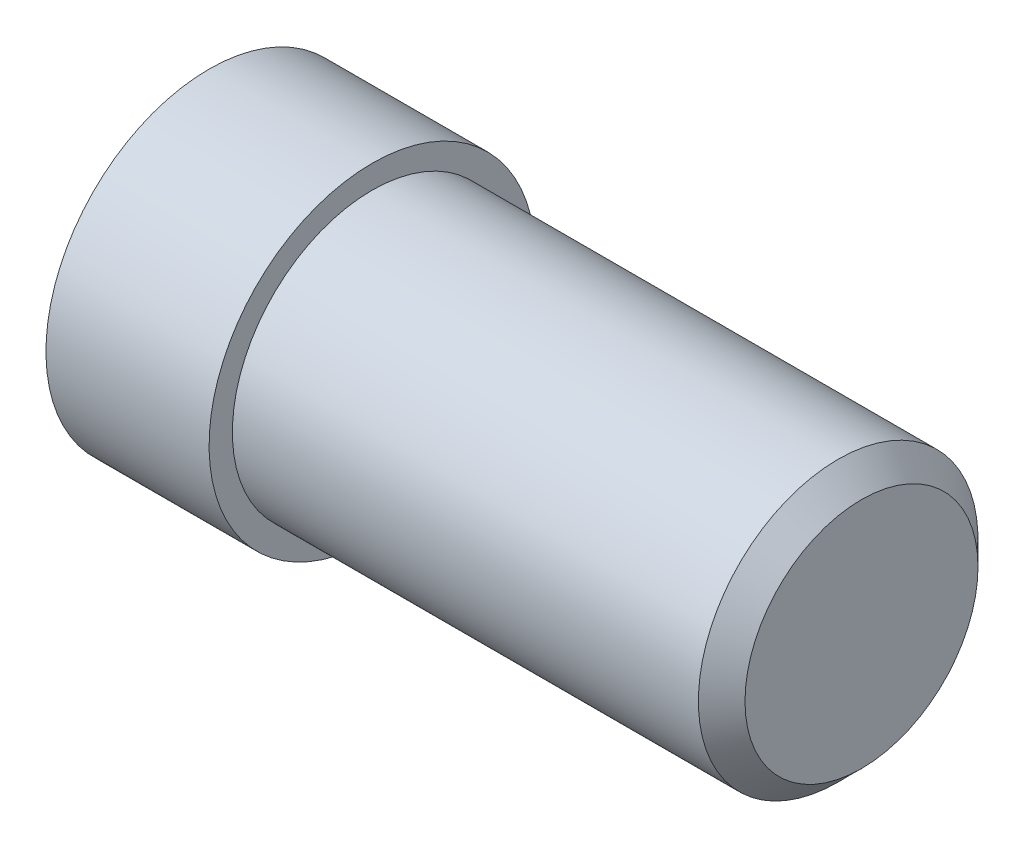
ISO-10303-21;
HEADER;
FILE_DESCRIPTION(('STEP AP214'),'2;1');
FILE_NAME('part.step','',(''),(''),'','','');
FILE_SCHEMA(('AUTOMOTIVE_DESIGN { 1 0 10303 214 1 1 1 1 }'));
ENDSEC;
DATA;
#1=APPLICATION_CONTEXT('core data for automotive mechanical design processes');
#2=APPLICATION_PROTOCOL_DEFINITION('international standard','automotive_design',2000,#1);
#3=PRODUCT_CONTEXT('',#1,'mechanical');
#4=PRODUCT('Part','Part','',(#3));
#5=PRODUCT_RELATED_PRODUCT_CATEGORY('part','',(#4));
#6=PRODUCT_DEFINITION_FORMATION('','',#4);
#7=PRODUCT_DEFINITION_CONTEXT('part definition',#1,'design');
#8=PRODUCT_DEFINITION('design','',#6,#7);
#9=PRODUCT_DEFINITION_SHAPE('','',#8);
#10=(LENGTH_UNIT() NAMED_UNIT(*) SI_UNIT(.MILLI.,.METRE.));
#11=(NAMED_UNIT(*) PLANE_ANGLE_UNIT() SI_UNIT($,.RADIAN.));
#12=(NAMED_UNIT(*) SI_UNIT($,.STERADIAN.) SOLID_ANGLE_UNIT());
#13=UNCERTAINTY_MEASURE_WITH_UNIT(LENGTH_MEASURE(1.E-05),#10,'distance_accuracy_value','');
#14=(GEOMETRIC_REPRESENTATION_CONTEXT(3) GLOBAL_UNCERTAINTY_ASSIGNED_CONTEXT((#13)) GLOBAL_UNIT_ASSIGNED_CONTEXT((#10,
#11,#12)) REPRESENTATION_CONTEXT('',''));
#15=CARTESIAN_POINT('',(0.,0.,0.));
#16=DIRECTION('',(0.,0.,1.));
#17=DIRECTION('',(1.,0.,0.));
#18=AXIS2_PLACEMENT_3D('',#15,#16,#17);
#19=CARTESIAN_POINT('',(0.,0.,0.));
#20=DIRECTION('',(1.,0.,0.));
#21=DIRECTION('',(0.,1.,0.));
#22=AXIS2_PLACEMENT_3D('',#19,#20,#21);
#23=PLANE('',#22);
#24=CARTESIAN_POINT('',(0.,0.,0.));
#25=DIRECTION('',(1.,0.,0.));
#26=DIRECTION('',(0.,1.,0.));
#27=AXIS2_PLACEMENT_3D('',#24,#25,#26);
#28=CIRCLE('',#27,5.);
#29=CARTESIAN_POINT('',(0.,5.,0.));
#30=VERTEX_POINT('',#29);
#31=EDGE_CURVE('E50',#30,#30,#28,.T.);
#32=ORIENTED_EDGE('',*,*,#31,.T.);
#33=EDGE_LOOP('',(#32));
#34=FACE_BOUND('',#33,.T.);
#35=ADVANCED_FACE('F39',(#34),#23,.T.);
#36=CARTESIAN_POINT('',(0.,0.,0.));
#37=DIRECTION('',(1.,0.,0.));
#38=DIRECTION('',(0.,1.,0.));
#39=AXIS2_PLACEMENT_3D('',#36,#37,#38);
#40=CYLINDRICAL_SURFACE('',#39,6.);
#41=CARTESIAN_POINT('',(-1.,0.,0.));
#42=DIRECTION('',(1.,0.,0.));
#43=DIRECTION('',(0.,1.,0.));
#44=AXIS2_PLACEMENT_3D('',#41,#42,#43);
#45=CIRCLE('',#44,6.);
#46=CARTESIAN_POINT('',(-1.,6.,0.));
#47=VERTEX_POINT('',#46);
#48=EDGE_CURVE('E10',#47,#47,#45,.F.);
#49=ORIENTED_EDGE('',*,*,#48,.T.);
#50=EDGE_LOOP('',(#49));
#51=FACE_BOUND('',#50,.T.);
#52=CARTESIAN_POINT('',(-21.,0.,0.));
#53=DIRECTION('',(1.,0.,0.));
#54=DIRECTION('',(0.,1.,0.));
#55=AXIS2_PLACEMENT_3D('',#52,#53,#54);
#56=CIRCLE('',#55,6.);
#57=CARTESIAN_POINT('',(-21.,5.99999999999999,0.));
#58=VERTEX_POINT('',#57);
#59=EDGE_CURVE('E51',#58,#58,#56,.T.);
#60=ORIENTED_EDGE('',*,*,#59,.T.);
#61=EDGE_LOOP('',(#60));
#62=FACE_BOUND('',#61,.T.);
#63=ADVANCED_FACE('F76',(#51,#62),#40,.T.);
#64=CARTESIAN_POINT('',(-21.,5.99999999999999,0.));
#65=DIRECTION('',(1.,0.,0.));
#66=DIRECTION('',(0.,1.,0.));
#67=AXIS2_PLACEMENT_3D('',#64,#65,#66);
#68=PLANE('',#67);
#69=CARTESIAN_POINT('',(-21.,0.,0.));
#70=DIRECTION('',(1.,0.,0.));
#71=DIRECTION('',(0.,1.,0.));
#72=AXIS2_PLACEMENT_3D('',#69,#70,#71);
#73=CIRCLE('',#72,7.);
#74=CARTESIAN_POINT('',(-21.,7.,0.));
#75=VERTEX_POINT('',#74);
#76=EDGE_CURVE('E54',#75,#75,#73,.T.);
#77=ORIENTED_EDGE('',*,*,#76,.T.);
#78=EDGE_LOOP('',(#77));
#79=FACE_BOUND('',#78,.T.);
#80=ORIENTED_EDGE('',*,*,#59,.F.);
#81=EDGE_LOOP('',(#80));
#82=FACE_BOUND('',#81,.T.);
#83=ADVANCED_FACE('F77',(#79,#82),#68,.T.);
#84=CARTESIAN_POINT('',(0.,0.,0.));
#85=DIRECTION('',(1.,0.,0.));
#86=DIRECTION('',(0.,1.,0.));
#87=AXIS2_PLACEMENT_3D('',#84,#85,#86);
#88=CYLINDRICAL_SURFACE('',#87,7.);
#89=CARTESIAN_POINT('',(-28.,0.,0.));
#90=DIRECTION('',(1.,0.,0.));
#91=DIRECTION('',(0.,1.,0.));
#92=AXIS2_PLACEMENT_3D('',#89,#90,#91);
#93=CIRCLE('',#92,7.);
#94=CARTESIAN_POINT('',(-28.,6.99999999999999,0.));
#95=VERTEX_POINT('',#94);
#96=EDGE_CURVE('E58',#95,#95,#93,.T.);
#97=ORIENTED_EDGE('',*,*,#96,.T.);
#98=EDGE_LOOP('',(#97));
#99=FACE_BOUND('',#98,.T.);
#100=ORIENTED_EDGE('',*,*,#76,.F.);
#101=EDGE_LOOP('',(#100));
#102=FACE_BOUND('',#101,.T.);
#103=ADVANCED_FACE('F61',(#99,#102),#88,.T.);
#104=CARTESIAN_POINT('',(-28.,6.99999999999999,0.));
#105=DIRECTION('',(-1.,0.,0.));
#106=DIRECTION('',(0.,-1.,0.));
#107=AXIS2_PLACEMENT_3D('',#104,#105,#106);
#108=PLANE('',#107);
#109=ORIENTED_EDGE('',*,*,#96,.F.);
#110=EDGE_LOOP('',(#109));
#111=FACE_BOUND('',#110,.T.);
#112=ADVANCED_FACE('F70',(#111),#108,.T.);
#113=CARTESIAN_POINT('',(0.,0.,0.));
#114=DIRECTION('',(-1.,0.,0.));
#115=DIRECTION('',(0.,-1.,0.));
#116=AXIS2_PLACEMENT_3D('',#113,#114,#115);
#117=CONICAL_SURFACE('',#116,5.,0.785398163397448);
#118=ORIENTED_EDGE('',*,*,#48,.F.);
#119=EDGE_LOOP('',(#118));
#120=FACE_BOUND('',#119,.T.);
#121=ORIENTED_EDGE('',*,*,#31,.F.);
#122=EDGE_LOOP('',(#121));
#123=FACE_BOUND('',#122,.T.);
#124=ADVANCED_FACE('F45',(#120,#123),#117,.T.);
#125=CLOSED_SHELL('',(#35,#63,#83,#103,#112,#124));
#126=MANIFOLD_SOLID_BREP('B2',#125);
#127=ADVANCED_BREP_SHAPE_REPRESENTATION('',(#18,#126),#14);
#128=SHAPE_DEFINITION_REPRESENTATION(#9,#127);
ENDSEC;
END-ISO-10303-21;
